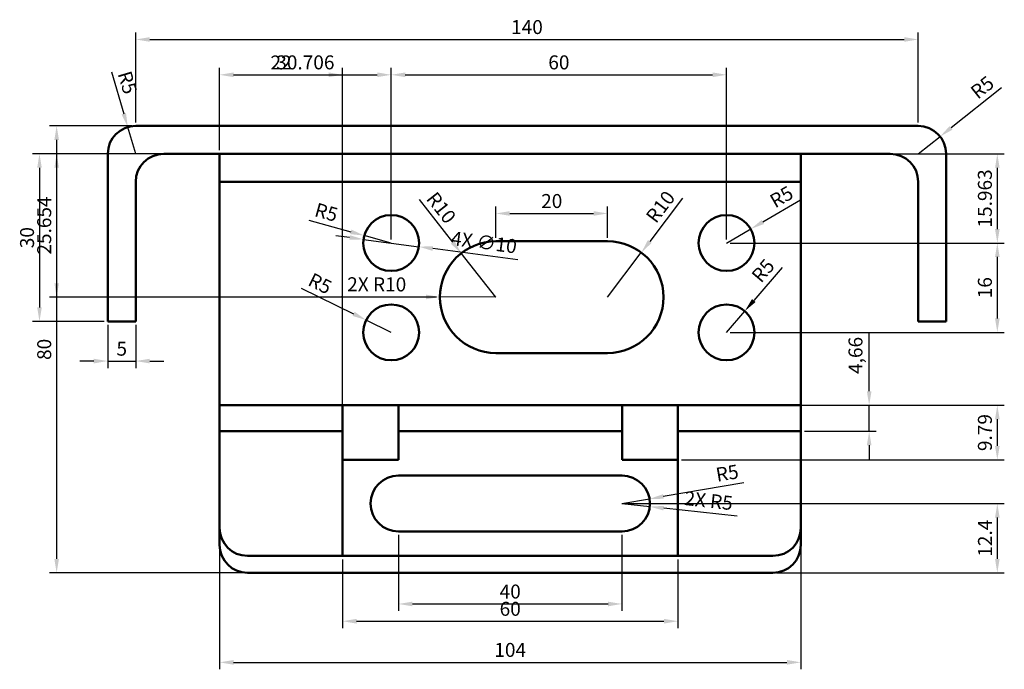
# Model space of a CAD drawing. Units: millimetres. Extents: x 1154 to 1562, y 1225 to 1481.
# Tile 2 of 4: x 1167 to 1343, y 1364 to 1481. Entities that reach past the tile are written whole.
import ezdxf

# ---------------------------------------------------------------- set-up
doc = ezdxf.new("R2010")
doc.units = ezdxf.units.MM
doc.layers.add('M-DIMS', color=2, linetype='Continuous', lineweight=25)
doc.layers.add('M-OUTL', color=7, linetype='Continuous', lineweight=50)
doc.styles.get("Standard").update_dxf_attribs({"font": 'arial.ttf'})
doc.dimstyles.new('ISO-25', dxfattribs={"dimtxt": 2.5, "dimasz": 2.5, "dimexe": 1.25, "dimexo": 0.625, "dimtad": 1, "dimtxsty": 'Standard', "dimcen": 2.5, "dimadec": 0, "dimazin": 0, "dimtfac": 1, "dimtmove": 0, "dimatfit": 3, "dimfxl": 1, "dimarcsym": 0})

# ---------------------------------------------------------------- blocks, each defined once
blk = doc.blocks.new('*D7')
at = {"layer": 'Defpoints', "color": 0, "transparency": 16777216}
for p in [(1234.3, 1389.02), (1274.3, 1389.02), (1274.3, 1376.05)]:
    blk.add_point(p, dxfattribs=at)
at = {"layer": 'M-DIMS', "color": 0, "lineweight": -2, "transparency": 16777216}
for p, q in [((1234.3, 1388.4), (1234.3, 1374.8)), ((1274.3, 1388.4), (1274.3, 1374.8)), ((1236.8, 1376.05), (1271.8, 1376.05))]:
    blk.add_line(p, q, dxfattribs=at)
at = {"layer": 'M-DIMS', "color": 0, "transparency": 16777216}
for points in [[(1236.8, 1376.46), (1236.8, 1375.63), (1234.3, 1376.05)], [(1271.8, 1376.46), (1271.8, 1375.63), (1274.3, 1376.05)]]:
    blk.add_solid(points, dxfattribs=at)
at = {"layer": 'M-DIMS', "color": 0, "transparency": 16777216, "insert": (1254.3, 1377.95), "char_height": 2.5, "attachment_point": 5}
blk.add_mtext('40', dxfattribs=at)
blk = doc.blocks.new('*D8')
at = {"layer": 'Defpoints', "color": 0, "transparency": 16777216}
for p in [(1224.3, 1384.66), (1284.3, 1384.66), (1284.3, 1372.96)]:
    blk.add_point(p, dxfattribs=at)
at = {"layer": 'M-DIMS', "color": 0, "lineweight": -2, "transparency": 16777216}
for p, q in [((1224.3, 1384.03), (1224.3, 1371.71)), ((1284.3, 1384.03), (1284.3, 1371.71)), ((1226.8, 1372.96), (1281.8, 1372.96))]:
    blk.add_line(p, q, dxfattribs=at)
at = {"layer": 'M-DIMS', "color": 0, "transparency": 16777216}
for points in [[(1226.8, 1373.38), (1226.8, 1372.54), (1224.3, 1372.96)], [(1281.8, 1373.38), (1281.8, 1372.54), (1284.3, 1372.96)]]:
    blk.add_solid(points, dxfattribs=at)
at = {"layer": 'M-DIMS', "color": 0, "transparency": 16777216, "insert": (1254.3, 1374.86), "char_height": 2.5, "attachment_point": 5}
blk.add_mtext('60', dxfattribs=at)
blk = doc.blocks.new('*D9')
at = {"layer": 'Defpoints', "color": 0, "transparency": 16777216}
for p in [(1271.73, 1445.95), (1251.73, 1440.97), (1271.73, 1440.97)]:
    blk.add_point(p, dxfattribs=at)
at = {"layer": 'M-DIMS', "color": 0, "lineweight": -2, "transparency": 16777216}
for p, q in [((1251.73, 1441.59), (1251.73, 1447.2)), ((1271.73, 1441.59), (1271.73, 1447.2)), ((1254.23, 1445.95), (1269.23, 1445.95))]:
    blk.add_line(p, q, dxfattribs=at)
at = {"layer": 'M-DIMS', "color": 0, "transparency": 16777216}
for points in [[(1254.23, 1446.36), (1254.23, 1445.53), (1251.73, 1445.95)], [(1269.23, 1446.36), (1269.23, 1445.53), (1271.73, 1445.95)]]:
    blk.add_solid(points, dxfattribs=at)
at = {"layer": 'M-DIMS', "color": 0, "transparency": 16777216, "insert": (1261.73, 1447.85), "char_height": 2.5, "attachment_point": 5}
blk.add_mtext('20', dxfattribs=at)
blk = doc.blocks.new('*D10')
at = {"layer": 'Defpoints', "color": 0, "transparency": 16777216}
for p in [(1277.76, 1438.94), (1271.73, 1430.97)]:
    blk.add_point(p, dxfattribs=at)
at = {"layer": 'M-DIMS', "color": 0, "lineweight": -2, "transparency": 16777216}
for p, q in [((1285.13, 1448.68), (1279.27, 1440.94)), ((1271.73, 1430.97), (1277.76, 1438.94))]:
    blk.add_line(p, q, dxfattribs=at)
at = {"layer": 'M-DIMS', "color": 0, "transparency": 16777216}
blk.add_solid([(1278.94, 1441.19), (1279.6, 1440.68), (1277.76, 1438.94)], dxfattribs=at)
at = {"layer": 'M-DIMS', "color": 0, "transparency": 16777216, "insert": (1281.44, 1446.95), "char_height": 2.5, "attachment_point": 5, "rotation": 52.8857}
blk.add_mtext('R10', dxfattribs=at)
blk = doc.blocks.new('*D11')
at = {"layer": 'Defpoints', "color": 0, "transparency": 16777216}
for p in [(1297.33, 1443.17), (1293.01, 1440.66)]:
    blk.add_point(p, dxfattribs=at)
at = {"layer": 'M-DIMS', "color": 0, "lineweight": -2, "transparency": 16777216}
for p, q in [((1306.24, 1448.34), (1299.49, 1444.42)), ((1293.01, 1440.66), (1297.33, 1443.17))]:
    blk.add_line(p, q, dxfattribs=at)
at = {"layer": 'M-DIMS', "color": 0, "transparency": 16777216}
blk.add_solid([(1299.29, 1444.78), (1299.7, 1444.06), (1297.33, 1443.17)], dxfattribs=at)
at = {"layer": 'M-DIMS', "color": 0, "transparency": 16777216, "insert": (1303, 1448.65), "char_height": 2.5, "attachment_point": 5, "rotation": 30.129}
blk.add_mtext('R5', dxfattribs=at)
blk = doc.blocks.new('*D12')
at = {"layer": 'Defpoints', "color": 0, "transparency": 16777216}
for p in [(1331.22, 1459.73), (1327.3, 1456.62)]:
    blk.add_point(p, dxfattribs=at)
at = {"layer": 'M-DIMS', "color": 0, "lineweight": -2, "transparency": 16777216}
for p, q in [((1342.21, 1468.43), (1333.18, 1461.28)), ((1327.3, 1456.62), (1331.22, 1459.73))]:
    blk.add_line(p, q, dxfattribs=at)
at = {"layer": 'M-DIMS', "color": 0, "transparency": 16777216}
blk.add_solid([(1332.92, 1461.6), (1333.44, 1460.95), (1331.22, 1459.73)], dxfattribs=at)
at = {"layer": 'M-DIMS', "color": 0, "transparency": 16777216, "insert": (1338.96, 1468.27), "char_height": 2.5, "attachment_point": 5, "rotation": 38.3673}
blk.add_mtext('R5', dxfattribs=at)
blk = doc.blocks.new('*D13')
at = {"layer": 'Defpoints', "color": 0, "transparency": 16777216}
for p in [(1182.3, 1456.62), (1170.08, 1426.62), (1182.3, 1426.62)]:
    blk.add_point(p, dxfattribs=at)
at = {"layer": 'M-DIMS', "color": 0, "lineweight": -2, "transparency": 16777216}
for p, q in [((1181.68, 1456.62), (1168.83, 1456.62)), ((1170.08, 1454.12), (1170.08, 1429.12)), ((1181.68, 1426.62), (1168.83, 1426.62))]:
    blk.add_line(p, q, dxfattribs=at)
at = {"layer": 'M-DIMS', "color": 0, "transparency": 16777216}
for points in [[(1169.67, 1454.12), (1170.5, 1454.12), (1170.08, 1456.62)], [(1169.67, 1429.12), (1170.5, 1429.12), (1170.08, 1426.62)]]:
    blk.add_solid(points, dxfattribs=at)
at = {"layer": 'M-DIMS', "color": 0, "transparency": 16777216, "insert": (1168.18, 1441.62), "char_height": 2.5, "attachment_point": 5, "rotation": 90}
blk.add_mtext('30', dxfattribs=at)
blk = doc.blocks.new('*D14')
at = {"layer": 'Defpoints', "color": 0, "transparency": 16777216}
for p in [(1182.3, 1426.62), (1187.3, 1426.62), (1187.3, 1419.53)]:
    blk.add_point(p, dxfattribs=at)
at = {"layer": 'M-DIMS', "color": 0, "lineweight": -2, "transparency": 16777216}
for p, q in [((1182.3, 1426), (1182.3, 1418.28)), ((1187.3, 1426), (1187.3, 1418.28)), ((1179.8, 1419.53), (1177.3, 1419.53)), ((1182.3, 1419.53), (1187.3, 1419.53)), ((1189.8, 1419.53), (1192.3, 1419.53))]:
    blk.add_line(p, q, dxfattribs=at)
at = {"layer": 'M-DIMS', "color": 0, "transparency": 16777216}
for points in [[(1179.8, 1419.94), (1179.8, 1419.11), (1182.3, 1419.53)], [(1189.8, 1419.94), (1189.8, 1419.11), (1187.3, 1419.53)]]:
    blk.add_solid(points, dxfattribs=at)
at = {"layer": 'M-DIMS', "color": 0, "transparency": 16777216, "insert": (1184.8, 1421.42), "char_height": 2.5, "attachment_point": 5}
blk.add_mtext('5', dxfattribs=at)
blk = doc.blocks.new('*D15')
at = {"layer": 'Defpoints', "color": 0, "transparency": 16777216}
for p in [(1327.3, 1477.09), (1187.3, 1461.62), (1327.3, 1461.62)]:
    blk.add_point(p, dxfattribs=at)
at = {"layer": 'M-DIMS', "color": 0, "lineweight": -2, "transparency": 16777216}
for p, q in [((1187.3, 1462.25), (1187.3, 1478.34)), ((1327.3, 1462.25), (1327.3, 1478.34)), ((1189.8, 1477.09), (1324.8, 1477.09))]:
    blk.add_line(p, q, dxfattribs=at)
at = {"layer": 'M-DIMS', "color": 0, "transparency": 16777216}
for points in [[(1189.8, 1477.51), (1189.8, 1476.68), (1187.3, 1477.09)], [(1324.8, 1477.51), (1324.8, 1476.68), (1327.3, 1477.09)]]:
    blk.add_solid(points, dxfattribs=at)
at = {"layer": 'M-DIMS', "color": 0, "transparency": 16777216, "insert": (1257.3, 1478.99), "char_height": 2.5, "attachment_point": 5}
blk.add_mtext('140', dxfattribs=at)
blk = doc.blocks.new('*D51')
at = {"layer": 'Defpoints', "color": 0, "transparency": 16777216}
for p in [(1306.3, 1411.62), (1318.52, 1411.62), (1306.3, 1406.96)]:
    blk.add_point(p, dxfattribs=at)
at = {"layer": 'M-DIMS', "color": 0, "lineweight": -2, "transparency": 16777216}
for p, q in [((1318.52, 1414.12), (1318.52, 1424.46)), ((1306.93, 1411.62), (1319.77, 1411.62)), ((1318.52, 1406.96), (1318.52, 1411.62)), ((1306.93, 1406.96), (1319.77, 1406.96)), ((1318.52, 1404.46), (1318.52, 1401.96))]:
    blk.add_line(p, q, dxfattribs=at)
at = {"layer": 'M-DIMS', "color": 0, "transparency": 16777216}
for points in [[(1318.11, 1414.12), (1318.94, 1414.12), (1318.52, 1411.62)], [(1318.11, 1404.46), (1318.94, 1404.46), (1318.52, 1406.96)]]:
    blk.add_solid(points, dxfattribs=at)
at = {"layer": 'M-DIMS', "color": 0, "transparency": 16777216, "insert": (1316.4, 1420.54), "char_height": 2.5, "attachment_point": 5, "rotation": 90}
blk.add_mtext('4,66', dxfattribs=at)
blk = doc.blocks.new('*D52')
at = {"layer": 'Defpoints', "color": 0, "transparency": 16777216}
for p in [(1202.3, 1388.14), (1306.3, 1386.62), (1306.3, 1365.6)]:
    blk.add_point(p, dxfattribs=at)
at = {"layer": 'M-DIMS', "color": 0, "lineweight": -2, "transparency": 16777216}
for p, q in [((1202.3, 1387.51), (1202.3, 1364.35)), ((1306.3, 1386), (1306.3, 1364.35)), ((1204.8, 1365.6), (1303.8, 1365.6))]:
    blk.add_line(p, q, dxfattribs=at)
at = {"layer": 'M-DIMS', "color": 0, "transparency": 16777216}
for points in [[(1204.8, 1366.02), (1204.8, 1365.18), (1202.3, 1365.6)], [(1303.8, 1366.02), (1303.8, 1365.18), (1306.3, 1365.6)]]:
    blk.add_solid(points, dxfattribs=at)
at = {"layer": 'M-DIMS', "color": 0, "transparency": 16777216, "insert": (1254.3, 1367.5), "char_height": 2.5, "attachment_point": 5}
blk.add_mtext('104', dxfattribs=at)
blk = doc.blocks.new('*D53')
at = {"layer": 'Defpoints', "color": 0, "transparency": 16777216}
for p in [(1274.3, 1394.02), (1279.23, 1394.86)]:
    blk.add_point(p, dxfattribs=at)
at = {"layer": 'M-DIMS', "color": 0, "lineweight": -2, "transparency": 16777216}
for p, q in [((1296.11, 1397.74), (1281.69, 1395.28)), ((1274.3, 1394.02), (1279.23, 1394.86))]:
    blk.add_line(p, q, dxfattribs=at)
at = {"layer": 'M-DIMS', "color": 0, "transparency": 16777216}
blk.add_solid([(1281.62, 1395.69), (1281.77, 1394.87), (1279.23, 1394.86)], dxfattribs=at)
at = {"layer": 'M-DIMS', "color": 0, "transparency": 16777216, "insert": (1293.18, 1399.16), "char_height": 2.5, "attachment_point": 5, "rotation": 9.6798}
blk.add_mtext('R5', dxfattribs=at)
blk = doc.blocks.new('*D54')
at = {"layer": 'Defpoints', "color": 0, "transparency": 16777216}
for p in [(1228.19, 1441.99), (1233.01, 1440.66)]:
    blk.add_point(p, dxfattribs=at)
at = {"layer": 'M-DIMS', "color": 0, "lineweight": -2, "transparency": 16777216}
for p, q in [((1218.26, 1444.73), (1225.78, 1442.66)), ((1233.01, 1440.66), (1228.19, 1441.99))]:
    blk.add_line(p, q, dxfattribs=at)
at = {"layer": 'M-DIMS', "color": 0, "transparency": 16777216}
blk.add_solid([(1225.89, 1443.06), (1225.67, 1442.25), (1228.19, 1441.99)], dxfattribs=at)
at = {"layer": 'M-DIMS', "color": 0, "transparency": 16777216, "insert": (1221.32, 1445.85), "char_height": 2.5, "attachment_point": 5, "rotation": 344.559}
blk.add_mtext('R5', dxfattribs=at)
blk = doc.blocks.new('*D55')
at = {"layer": 'Defpoints', "color": 0, "transparency": 16777216}
for p in [(1228.52, 1426.87), (1233.01, 1424.66)]:
    blk.add_point(p, dxfattribs=at)
at = {"layer": 'M-DIMS', "color": 0, "lineweight": -2, "transparency": 16777216}
for p, q in [((1216.92, 1432.59), (1226.28, 1427.98)), ((1233.01, 1424.66), (1228.52, 1426.87))]:
    blk.add_line(p, q, dxfattribs=at)
at = {"layer": 'M-DIMS', "color": 0, "transparency": 16777216}
blk.add_solid([(1226.47, 1428.35), (1226.1, 1427.6), (1228.52, 1426.87)], dxfattribs=at)
at = {"layer": 'M-DIMS', "color": 0, "transparency": 16777216, "insert": (1220.14, 1433.12), "char_height": 2.5, "attachment_point": 5, "rotation": 333.7363}
blk.add_mtext('R5', dxfattribs=at)
blk = doc.blocks.new('*D56')
at = {"layer": 'Defpoints', "color": 0, "transparency": 16777216}
for p in [(1296.26, 1428.46), (1293.01, 1424.66)]:
    blk.add_point(p, dxfattribs=at)
at = {"layer": 'M-DIMS', "color": 0, "lineweight": -2, "transparency": 16777216}
for p, q in [((1302.95, 1436.29), (1297.88, 1430.36)), ((1293.01, 1424.66), (1296.26, 1428.46))]:
    blk.add_line(p, q, dxfattribs=at)
at = {"layer": 'M-DIMS', "color": 0, "transparency": 16777216}
blk.add_solid([(1297.56, 1430.63), (1298.2, 1430.09), (1296.26, 1428.46)], dxfattribs=at)
at = {"layer": 'M-DIMS', "color": 0, "transparency": 16777216, "insert": (1299.78, 1435.51), "char_height": 2.5, "attachment_point": 5, "rotation": 49.4858}
blk.add_mtext('R5', dxfattribs=at)
blk = doc.blocks.new('*D57')
at = {"layer": 'Defpoints', "color": 0, "transparency": 16777216}
for p in [(1245.54, 1438.83), (1251.73, 1430.97)]:
    blk.add_point(p, dxfattribs=at)
at = {"layer": 'M-DIMS', "color": 0, "lineweight": -2, "transparency": 16777216}
for p, q in [((1237.99, 1448.43), (1244, 1440.79)), ((1251.73, 1430.97), (1245.54, 1438.83))]:
    blk.add_line(p, q, dxfattribs=at)
at = {"layer": 'M-DIMS', "color": 0, "transparency": 16777216}
blk.add_solid([(1244.32, 1441.05), (1243.67, 1440.53), (1245.54, 1438.83)], dxfattribs=at)
at = {"layer": 'M-DIMS', "color": 0, "transparency": 16777216, "insert": (1241.71, 1446.77), "char_height": 2.5, "attachment_point": 5, "rotation": 308.1956}
blk.add_mtext('R10', dxfattribs=at)
blk = doc.blocks.new('*D68')
at = {"layer": 'Defpoints', "color": 0, "transparency": 16777216}
for p in [(1187.3, 1461.62), (1173.15, 1381.62), (1207.3, 1381.62)]:
    blk.add_point(p, dxfattribs=at)
at = {"layer": 'M-DIMS', "color": 0, "lineweight": -2, "transparency": 16777216}
for p, q in [((1186.68, 1461.62), (1171.9, 1461.62)), ((1173.15, 1459.12), (1173.15, 1384.12)), ((1206.68, 1381.62), (1171.9, 1381.62))]:
    blk.add_line(p, q, dxfattribs=at)
at = {"layer": 'M-DIMS', "color": 0, "transparency": 16777216}
for points in [[(1172.74, 1459.12), (1173.57, 1459.12), (1173.15, 1461.62)], [(1172.74, 1384.12), (1173.57, 1384.12), (1173.15, 1381.62)]]:
    blk.add_solid(points, dxfattribs=at)
at = {"layer": 'M-DIMS', "color": 0, "transparency": 16777216, "insert": (1171.25, 1421.62), "char_height": 2.5, "attachment_point": 5, "rotation": 90}
blk.add_mtext('80', dxfattribs=at)
blk = doc.blocks.new('*D69')
at = {"layer": 'Defpoints', "color": 0, "transparency": 16777216}
for p in [(1293.01, 1470.77), (1233.01, 1440.66), (1293.01, 1440.66)]:
    blk.add_point(p, dxfattribs=at)
at = {"layer": 'M-DIMS', "color": 0, "lineweight": -2, "transparency": 16777216}
for p, q in [((1233.01, 1441.28), (1233.01, 1472.02)), ((1293.01, 1441.28), (1293.01, 1472.02)), ((1235.51, 1470.77), (1290.51, 1470.77))]:
    blk.add_line(p, q, dxfattribs=at)
at = {"layer": 'M-DIMS', "color": 0, "transparency": 16777216}
for points in [[(1235.51, 1471.19), (1235.51, 1470.35), (1233.01, 1470.77)], [(1290.51, 1471.19), (1290.51, 1470.35), (1293.01, 1470.77)]]:
    blk.add_solid(points, dxfattribs=at)
at = {"layer": 'M-DIMS', "color": 0, "transparency": 16777216, "insert": (1263.01, 1472.67), "char_height": 2.5, "attachment_point": 5}
blk.add_mtext('60', dxfattribs=at)
blk = doc.blocks.new('*D70')
at = {"layer": 'Defpoints', "color": 0, "transparency": 16777216}
for p in [(1293.01, 1440.66), (1293.01, 1424.66), (1341.45, 1424.66)]:
    blk.add_point(p, dxfattribs=at)
at = {"layer": 'M-DIMS', "color": 0, "lineweight": -2, "transparency": 16777216}
for p, q in [((1293.63, 1440.66), (1342.7, 1440.66)), ((1341.45, 1438.16), (1341.45, 1427.16)), ((1293.63, 1424.66), (1342.7, 1424.66))]:
    blk.add_line(p, q, dxfattribs=at)
at = {"layer": 'M-DIMS', "color": 0, "transparency": 16777216}
for points in [[(1341.04, 1438.16), (1341.87, 1438.16), (1341.45, 1440.66)], [(1341.04, 1427.16), (1341.87, 1427.16), (1341.45, 1424.66)]]:
    blk.add_solid(points, dxfattribs=at)
at = {"layer": 'M-DIMS', "color": 0, "transparency": 16777216, "insert": (1339.55, 1432.66), "char_height": 2.5, "attachment_point": 5, "rotation": 90}
blk.add_mtext('16', dxfattribs=at)
blk = doc.blocks.new('*D71')
at = {"layer": 'Defpoints', "color": 0, "transparency": 16777216}
for p in [(1233.01, 1470.77), (1202.3, 1456.62), (1233.01, 1440.66)]:
    blk.add_point(p, dxfattribs=at)
at = {"layer": 'M-DIMS', "color": 0, "lineweight": -2, "transparency": 16777216}
for p, q in [((1202.3, 1457.25), (1202.3, 1472.02)), ((1233.01, 1441.28), (1233.01, 1472.02)), ((1204.8, 1470.77), (1230.51, 1470.77))]:
    blk.add_line(p, q, dxfattribs=at)
at = {"layer": 'M-DIMS', "color": 0, "transparency": 16777216}
for points in [[(1204.8, 1471.19), (1204.8, 1470.35), (1202.3, 1470.77)], [(1230.51, 1471.19), (1230.51, 1470.35), (1233.01, 1470.77)]]:
    blk.add_solid(points, dxfattribs=at)
at = {"layer": 'M-DIMS', "color": 0, "transparency": 16777216, "insert": (1217.65, 1472.67), "char_height": 2.5, "attachment_point": 5}
blk.add_mtext('30.706', dxfattribs=at)
blk = doc.blocks.new('*D72')
at = {"layer": 'Defpoints', "color": 0, "transparency": 16777216}
for p in [(1306.3, 1456.62), (1293.01, 1440.66), (1341.45, 1440.66)]:
    blk.add_point(p, dxfattribs=at)
at = {"layer": 'M-DIMS', "color": 0, "lineweight": -2, "transparency": 16777216}
for p, q in [((1306.93, 1456.62), (1342.7, 1456.62)), ((1341.45, 1454.12), (1341.45, 1443.16)), ((1293.63, 1440.66), (1342.7, 1440.66))]:
    blk.add_line(p, q, dxfattribs=at)
at = {"layer": 'M-DIMS', "color": 0, "transparency": 16777216}
for points in [[(1341.04, 1454.12), (1341.87, 1454.12), (1341.45, 1456.62)], [(1341.04, 1443.16), (1341.87, 1443.16), (1341.45, 1440.66)]]:
    blk.add_solid(points, dxfattribs=at)
at = {"layer": 'M-DIMS', "color": 0, "transparency": 16777216, "insert": (1339.55, 1448.64), "char_height": 2.5, "attachment_point": 5, "rotation": 90}
blk.add_mtext('15.963', dxfattribs=at)
blk = doc.blocks.new('*D73')
at = {"layer": 'Defpoints', "color": 0, "transparency": 16777216}
for p in [(1202.3, 1456.62), (1173.15, 1430.97), (1241.73, 1430.97)]:
    blk.add_point(p, dxfattribs=at)
at = {"layer": 'M-DIMS', "color": 0, "lineweight": -2, "transparency": 16777216}
for p, q in [((1201.68, 1456.62), (1171.9, 1456.62)), ((1173.15, 1454.12), (1173.15, 1433.47)), ((1241.1, 1430.97), (1171.9, 1430.97))]:
    blk.add_line(p, q, dxfattribs=at)
at = {"layer": 'M-DIMS', "color": 0, "transparency": 16777216}
for points in [[(1172.74, 1454.12), (1173.57, 1454.12), (1173.15, 1456.62)], [(1172.74, 1433.47), (1173.57, 1433.47), (1173.15, 1430.97)]]:
    blk.add_solid(points, dxfattribs=at)
at = {"layer": 'M-DIMS', "color": 0, "transparency": 16777216, "insert": (1171.25, 1443.79), "char_height": 2.5, "attachment_point": 5, "rotation": 90}
blk.add_mtext('25.654', dxfattribs=at)
blk = doc.blocks.new('*D74')
at = {"layer": 'Defpoints', "color": 0, "transparency": 16777216}
for p in [(1284.3, 1411.62), (1284.3, 1401.83), (1341.45, 1401.83)]:
    blk.add_point(p, dxfattribs=at)
at = {"layer": 'M-DIMS', "color": 0, "lineweight": -2, "transparency": 16777216}
for p, q in [((1284.93, 1411.62), (1342.7, 1411.62)), ((1341.45, 1409.12), (1341.45, 1404.33)), ((1284.93, 1401.83), (1342.7, 1401.83))]:
    blk.add_line(p, q, dxfattribs=at)
at = {"layer": 'M-DIMS', "color": 0, "transparency": 16777216}
for points in [[(1341.04, 1409.12), (1341.87, 1409.12), (1341.45, 1411.62)], [(1341.04, 1404.33), (1341.87, 1404.33), (1341.45, 1401.83)]]:
    blk.add_solid(points, dxfattribs=at)
at = {"layer": 'M-DIMS', "color": 0, "transparency": 16777216, "insert": (1339.55, 1406.73), "char_height": 2.5, "attachment_point": 5, "rotation": 90}
blk.add_mtext('9.79', dxfattribs=at)
blk = doc.blocks.new('*D75')
at = {"layer": 'Defpoints', "color": 0, "transparency": 16777216}
for p in [(1274.3, 1394.02), (1301.3, 1381.62), (1341.45, 1381.62)]:
    blk.add_point(p, dxfattribs=at)
at = {"layer": 'M-DIMS', "color": 0, "lineweight": -2, "transparency": 16777216}
for p, q in [((1274.93, 1394.02), (1342.7, 1394.02)), ((1341.45, 1391.52), (1341.45, 1384.12)), ((1301.93, 1381.62), (1342.7, 1381.62))]:
    blk.add_line(p, q, dxfattribs=at)
at = {"layer": 'M-DIMS', "color": 0, "transparency": 16777216}
for points in [[(1341.04, 1391.52), (1341.87, 1391.52), (1341.45, 1394.02)], [(1341.04, 1384.12), (1341.87, 1384.12), (1341.45, 1381.62)]]:
    blk.add_solid(points, dxfattribs=at)
at = {"layer": 'M-DIMS', "color": 0, "transparency": 16777216, "insert": (1339.57, 1387.82), "char_height": 2.5, "attachment_point": 5, "rotation": 90}
blk.add_mtext('12.4', dxfattribs=at)
blk = doc.blocks.new('*D76')
at = {"layer": 'Defpoints', "color": 0, "transparency": 16777216}
for p in [(1224.3, 1470.77), (1202.3, 1456.62), (1224.3, 1401.83)]:
    blk.add_point(p, dxfattribs=at)
at = {"layer": 'M-DIMS', "color": 0, "lineweight": -2, "transparency": 16777216}
for p, q in [((1202.3, 1457.25), (1202.3, 1472.02)), ((1224.3, 1402.46), (1224.3, 1472.02)), ((1204.8, 1470.77), (1221.8, 1470.77))]:
    blk.add_line(p, q, dxfattribs=at)
at = {"layer": 'M-DIMS', "color": 0, "transparency": 16777216}
for points in [[(1204.8, 1471.19), (1204.8, 1470.35), (1202.3, 1470.77)], [(1221.8, 1471.19), (1221.8, 1470.35), (1224.3, 1470.77)]]:
    blk.add_solid(points, dxfattribs=at)
at = {"layer": 'M-DIMS', "color": 0, "transparency": 16777216, "insert": (1213.3, 1472.65), "char_height": 2.5, "attachment_point": 5}
blk.add_mtext('22', dxfattribs=at)
blk = doc.blocks.new('*D95')
at = {"layer": 'Defpoints', "color": 0, "transparency": 16777216}
for p in [(1228.05, 1441.31), (1237.96, 1440)]:
    blk.add_point(p, dxfattribs=at)
at = {"layer": 'M-DIMS', "color": 0, "lineweight": -2, "transparency": 16777216}
for p, q in [((1225.57, 1441.64), (1223.09, 1441.97)), ((1228.05, 1441.31), (1237.96, 1440)), ((1255.69, 1437.66), (1240.44, 1439.68))]:
    blk.add_line(p, q, dxfattribs=at)
at = {"layer": 'M-DIMS', "color": 0, "transparency": 16777216}
for points in [[(1225.63, 1442.05), (1225.52, 1441.23), (1228.05, 1441.31)], [(1240.5, 1440.09), (1240.39, 1439.26), (1237.96, 1440)]]:
    blk.add_solid(points, dxfattribs=at)
at = {"layer": 'M-DIMS', "color": 0, "transparency": 16777216, "insert": (1249.57, 1440.46), "char_height": 2.5, "attachment_point": 5, "rotation": 352.4813}
blk.add_mtext('4X ∅10', dxfattribs=at)
blk = doc.blocks.new('*D96')
at = {"layer": 'Defpoints', "color": 0, "transparency": 16777216}
for p in [(1241.73, 1431), (1251.73, 1430.97)]:
    blk.add_point(p, dxfattribs=at)
at = {"layer": 'M-DIMS', "color": 0, "lineweight": -2, "transparency": 16777216}
for p, q in [((1224.1, 1431.06), (1239.23, 1431.01)), ((1251.73, 1430.97), (1241.73, 1431))]:
    blk.add_line(p, q, dxfattribs=at)
at = {"layer": 'M-DIMS', "color": 0, "transparency": 16777216}
blk.add_solid([(1239.23, 1431.42), (1239.22, 1430.59), (1241.73, 1431)], dxfattribs=at)
at = {"layer": 'M-DIMS', "color": 0, "transparency": 16777216, "insert": (1230.42, 1432.94), "char_height": 2.5, "attachment_point": 5, "rotation": 359.8142}
blk.add_mtext('2X R10', dxfattribs=at)
blk = doc.blocks.new('*D97')
at = {"layer": 'Defpoints', "color": 0, "transparency": 16777216}
for p in [(1274.3, 1394.02), (1279.27, 1393.47)]:
    blk.add_point(p, dxfattribs=at)
at = {"layer": 'M-DIMS', "color": 0, "lineweight": -2, "transparency": 16777216}
for p, q in [((1274.3, 1394.02), (1279.27, 1393.47)), ((1294.89, 1391.74), (1281.76, 1393.19))]:
    blk.add_line(p, q, dxfattribs=at)
at = {"layer": 'M-DIMS', "color": 0, "transparency": 16777216}
blk.add_solid([(1281.8, 1393.61), (1281.71, 1392.78), (1279.27, 1393.47)], dxfattribs=at)
at = {"layer": 'M-DIMS', "color": 0, "transparency": 16777216, "insert": (1289.77, 1394.22), "char_height": 2.5, "attachment_point": 5, "rotation": 353.678}
blk.add_mtext('2X R5', dxfattribs=at)
blk = doc.blocks.new('*D98')
at = {"layer": 'Defpoints', "color": 0, "transparency": 16777216}
for p in [(1185.88, 1461.41), (1187.3, 1456.62)]:
    blk.add_point(p, dxfattribs=at)
at = {"layer": 'M-DIMS', "color": 0, "lineweight": -2, "transparency": 16777216}
for p, q in [((1182.94, 1471.29), (1185.16, 1463.81)), ((1187.3, 1456.62), (1185.88, 1461.41))]:
    blk.add_line(p, q, dxfattribs=at)
at = {"layer": 'M-DIMS', "color": 0, "transparency": 16777216}
blk.add_solid([(1185.56, 1463.93), (1184.77, 1463.69), (1185.88, 1461.41)], dxfattribs=at)
at = {"layer": 'M-DIMS', "color": 0, "transparency": 16777216, "insert": (1185.51, 1469.29), "char_height": 2.5, "attachment_point": 5, "rotation": 286.5575}
blk.add_mtext('R5', dxfattribs=at)

msp = doc.modelspace()

# ---------------------------------------------------------------- linework, layer by layer
at = {"layer": 'M-OUTL'}
for p, q in [((1202.3017, 1461.6216), (1187.3017, 1461.6216)), ((1202.3017, 1461.6216), (1306.3017, 1461.6216)), ((1327.3017, 1461.6216), (1306.3017, 1461.6216)), ((1182.3017, 1456.6216), (1182.3017, 1426.6216)), ((1192.3017, 1456.6216), (1322.3017, 1456.6216)), ((1202.3017, 1389.6569), (1202.3017, 1456.6216)), ((1202.3017, 1456.6216), (1202.3017, 1451.6216)), ((1306.3017, 1456.6216), (1306.3017, 1389.6569)), ((1332.3017, 1426.6216), (1332.3017, 1456.6216)), ((1187.3017, 1426.6216), (1187.3017, 1451.6216)), ((1202.3017, 1451.6216), (1306.3017, 1451.6216)), ((1202.3017, 1451.6216), (1202.3017, 1411.6216)), ((1327.3017, 1451.6216), (1327.3017, 1426.6216)), ((1271.7255, 1440.9675), (1251.7255, 1440.9675)), ((1202.3017, 1421.6216), (1202.3017, 1431.6216)), ((1182.3017, 1426.6216), (1187.3017, 1426.6216)), ((1327.3017, 1426.6216), (1332.3017, 1426.6216)), ((1251.7255, 1420.9675), (1271.7255, 1420.9675)), ((1202.3017, 1411.6216), (1306.3017, 1411.6216)), ((1254.3017, 1411.6216), (1224.3017, 1411.6216)), ((1224.3017, 1411.6216), (1234.3017, 1411.6216)), ((1224.3017, 1411.6216), (1224.3017, 1401.8311)), ((1234.3017, 1411.6216), (1234.3017, 1401.8311)), ((1284.3017, 1411.6216), (1274.3017, 1411.6216)), ((1274.3017, 1411.6216), (1274.3017, 1401.8311)), ((1284.3017, 1384.6569), (1284.3017, 1411.6216)), ((1202.3017, 1406.9571), (1224.3017, 1406.9571)), ((1234.3017, 1406.9571), (1274.3017, 1406.9571)), ((1284.3017, 1406.9571), (1306.3017, 1406.9571)), ((1224.3017, 1401.8311), (1234.3017, 1401.8311)), ((1224.3017, 1401.8311), (1224.3017, 1384.6569)), ((1274.3017, 1401.8311), (1284.3017, 1401.8311)), ((1234.3017, 1399.0205), (1274.3017, 1399.0205)), ((1202.3017, 1386.6216), (1202.3017, 1389.6569)), ((1274.3017, 1389.0205), (1234.3017, 1389.0205)), ((1306.3017, 1386.6216), (1306.3017, 1389.6569)), ((1301.3017, 1384.6569), (1207.3017, 1384.6569)), ((1301.3017, 1381.6216), (1207.3017, 1381.6216))]:
    msp.add_line(p, q, dxfattribs=at)
for centre in [(1233.0076, 1440.6589), (1293.0076, 1440.6589), (1233.0076, 1424.6589), (1293.0076, 1424.6589)]:
    msp.add_circle(centre, 5, dxfattribs=at)
for centre, radius, start, end in [((1187.3017, 1456.6216), 5, 90, 180), ((1327.3017, 1456.6216), 5, 0, 90), ((1192.3017, 1451.6216), 5, 90, 180), ((1322.3017, 1451.6216), 5, 0, 90), ((1251.7255, 1430.9675), 10, 90, 270), ((1271.7255, 1430.9675), 10, 270, 90), ((1234.3017, 1394.0205), 5, 90, 270), ((1274.3017, 1394.0205), 5, 270, 90), ((1207.3017, 1389.6569), 5, 180, 270), ((1301.3017, 1389.6569), 5, 270, 0), ((1207.3017, 1386.6216), 5, 180, 270), ((1301.3017, 1386.6216), 5, 270, 0)]:
    msp.add_arc(centre, radius, start, end, dxfattribs=at)

# ---------------------------------------------------------------- dimensions: what is measured, and where the dimension line sits
at = {"layer": 'M-DIMS'}
for base, p1, p2, override, picture, middle in [((1327.3017, 1477.0928), (1187.3017, 1461.6216), (1327.3017, 1461.6216), {"dimclrd": 0, "dimclre": 0, "dimclrt": 0}, '*D15', (1257.3017, 1478.9942)), ((1233.0076, 1470.7716), (1202.3017, 1456.6216), (1233.0076, 1440.6589), {"dimdec": 3, "dimlfac": 1, "dimrnd": 0, "dimzin": 0, "dimdsep": 46, "dimlunit": 2}, '*D71', (1217.6547, 1472.6739)), ((1224.3017, 1470.7716), (1202.3017, 1456.6216), (1224.3017, 1401.8311), {"dimdec": 0, "dimlfac": 1, "dimrnd": 0, "dimzin": 0, "dimdsep": 46, "dimlunit": 2}, '*D76', (1213.3017, 1472.6517)), ((1293.0076, 1470.7716), (1233.0076, 1440.6589), (1293.0076, 1440.6589), {"dimdec": 0, "dimlfac": 1, "dimrnd": 0, "dimzin": 0, "dimdsep": 46, "dimlunit": 2}, '*D69', (1263.0076, 1472.673)), ((1271.7255, 1445.947), (1251.7255, 1440.9675), (1271.7255, 1440.9675), {"dimclrd": 0, "dimclre": 0, "dimclrt": 0}, '*D9', (1261.7255, 1447.8484)), ((1187.3017, 1419.5268), (1182.3017, 1426.6216), (1187.3017, 1426.6216), {"dimclrd": 0, "dimclre": 0, "dimclrt": 0}, '*D14', (1184.8017, 1421.4231)), ((1274.3017, 1376.0483), (1234.3017, 1389.0205), (1274.3017, 1389.0205), {"dimclrd": 0, "dimclre": 0, "dimclrt": 0}, '*D7', (1254.3017, 1377.9497)), ((1306.3017, 1365.6012), (1202.3017, 1388.1393), (1306.3017, 1386.6216), {"dimclrd": 0, "dimclre": 0, "dimclrt": 0}, '*D52', (1254.3017, 1367.5026)), ((1284.3017, 1372.9599), (1224.3017, 1384.6569), (1284.3017, 1384.6569), {"dimclrd": 0, "dimclre": 0, "dimclrt": 0}, '*D8', (1254.3017, 1374.8614))]:
    dim = msp.add_linear_dim(base=base, p1=p1, p2=p2, dimstyle='ISO-25', override=override, dxfattribs=at)
    dim.commit()
    dim.dimension.update_dxf_attribs({"geometry": picture, "text_midpoint": middle})
for center, mpoint, override, picture, middle in [((1187.3017, 1456.6216), (1185.8768, 1461.4143), {"dimdec": 0, "dimlfac": 1, "dimrnd": 0, "dimzin": 0, "dimdsep": 46, "dimlunit": 2}, '*D98', (1185.5144, 1469.2875)), ((1251.7255, 1430.9675), (1245.542, 1438.8265), {"dimclrd": 0, "dimclre": 0, "dimclrt": 0}, '*D57', (1241.7139, 1446.767)), ((1271.7255, 1430.9675), (1277.7596, 1438.9418), {"dimclrd": 0, "dimclre": 0, "dimclrt": 0}, '*D10', (1281.4372, 1446.9531)), ((1293.0076, 1440.6589), (1297.3321, 1443.1687), {"dimclrd": 0, "dimclre": 0, "dimclrt": 0}, '*D11', (1302.9968, 1448.6487)), ((1233.0076, 1440.6589), (1228.1881, 1441.9901), {"dimclrd": 0, "dimclre": 0, "dimclrt": 0}, '*D54', (1221.3191, 1445.8548)), ((1293.0076, 1424.6589), (1296.2558, 1428.4601), {"dimclrd": 0, "dimclre": 0, "dimclrt": 0}, '*D56', (1299.7839, 1435.508))]:
    dim = msp.add_radius_dim(center=center, mpoint=mpoint, dimstyle='ISO-25', override=override, dxfattribs=at)
    dim.commit()
    dim.dimension.update_dxf_attribs({"geometry": picture, "text_midpoint": middle})
for center, mpoint, picture, middle in [((1327.3017, 1456.6216), (1331.222, 1459.7251), '*D12', (1340.1366, 1466.7824)), ((1233.0076, 1424.6589), (1228.5238, 1426.8714), '*D55', (1219.3012, 1431.4223)), ((1274.3017, 1394.0205), (1279.2305, 1394.8612), '*D53', (1293.4998, 1397.2951))]:
    dim = msp.add_radius_dim(center=center, mpoint=mpoint, dimstyle='ISO-25', override={"dimclrd": 0, "dimclre": 0, "dimclrt": 0}, dxfattribs=at)
    dim.commit()
    dim.dimension.update_dxf_attribs({"geometry": picture, "text_midpoint": middle, "dimtype": 164})
for base, p1, p2, override, picture, middle in [((1173.1517, 1381.6216), (1187.3017, 1461.6216), (1207.3017, 1381.6216), {"dimdec": 0, "dimlfac": 1, "dimrnd": 0, "dimzin": 0, "dimdsep": 46, "dimlunit": 2}, '*D68', (1171.2503, 1421.6216)), ((1170.0825, 1426.6216), (1182.3017, 1456.6216), (1182.3017, 1426.6216), {"dimclrd": 0, "dimclre": 0, "dimclrt": 0}, '*D13', (1168.1802, 1441.6216)), ((1173.1517, 1430.9675), (1202.3017, 1456.6216), (1241.7255, 1430.9675), {"dimdec": 3, "dimlfac": 1, "dimrnd": 0, "dimzin": 0, "dimdsep": 46, "dimlunit": 2}, '*D73', (1171.2503, 1443.7945)), ((1341.4517, 1440.6589), (1306.3017, 1456.6216), (1293.0076, 1440.6589), {"dimdec": 3, "dimlfac": 1, "dimrnd": 0, "dimzin": 0, "dimdsep": 46, "dimlunit": 2}, '*D72', (1339.5494, 1448.6403)), ((1341.4517, 1424.6589), (1293.0076, 1440.6589), (1293.0076, 1424.6589), {"dimdec": 0, "dimlfac": 1, "dimrnd": 0, "dimzin": 0, "dimdsep": 46, "dimlunit": 2}, '*D70', (1339.5503, 1432.6589)), ((1318.5233, 1411.6216), (1306.3017, 1406.9571), (1306.3017, 1411.6216), {"dimclrd": 0, "dimclre": 0, "dimclrt": 0}, '*D51', (1316.3959, 1420.543)), ((1341.4517, 1401.8311), (1284.3017, 1411.6216), (1284.3017, 1401.8311), {"dimdec": 2, "dimlfac": 1, "dimrnd": 0, "dimzin": 0, "dimdsep": 46, "dimlunit": 2}, '*D74', (1339.5503, 1406.7263)), ((1341.4517, 1381.6216), (1274.3017, 1394.0205), (1301.3017, 1381.6216), {"dimdec": 1, "dimlfac": 1, "dimrnd": 0, "dimzin": 0, "dimdsep": 46, "dimlunit": 2}, '*D75', (1339.5716, 1387.8211))]:
    dim = msp.add_linear_dim(base=base, p1=p1, p2=p2, angle=90, dimstyle='ISO-25', override=override, dxfattribs=at)
    dim.commit()
    dim.dimension.update_dxf_attribs({"geometry": picture, "text_midpoint": middle})
dim = msp.add_diameter_dim_2p(p1=(1228.0506, 1441.3132), p2=(1237.9646, 1440.0047), text='4X <>', dimstyle='ISO-25', override={"dimdec": 0, "dimlfac": 1, "dimrnd": 0, "dimzin": 0, "dimdsep": 46, "dimlunit": 2}, dxfattribs=at)
dim.commit()
dim.dimension.update_dxf_attribs({"geometry": '*D95', "text_midpoint": (1249.3073, 1438.5076), "dimtype": 163})
for center, mpoint, picture, middle in [((1251.7255, 1430.9675), (1241.7256, 1430.9999), '*D96', (1230.417, 1432.938)), ((1274.3017, 1394.0205), (1279.2713, 1393.4699), '*D97', (1289.775, 1394.2193))]:
    dim = msp.add_radius_dim(center=center, mpoint=mpoint, text='2X <>', dimstyle='ISO-25', override={"dimdec": 0, "dimlfac": 1, "dimrnd": 0, "dimzin": 0, "dimdsep": 46, "dimlunit": 2}, dxfattribs=at)
    dim.commit()
    dim.dimension.update_dxf_attribs({"geometry": picture, "text_midpoint": middle})

doc.saveas('drawing.dxf')
